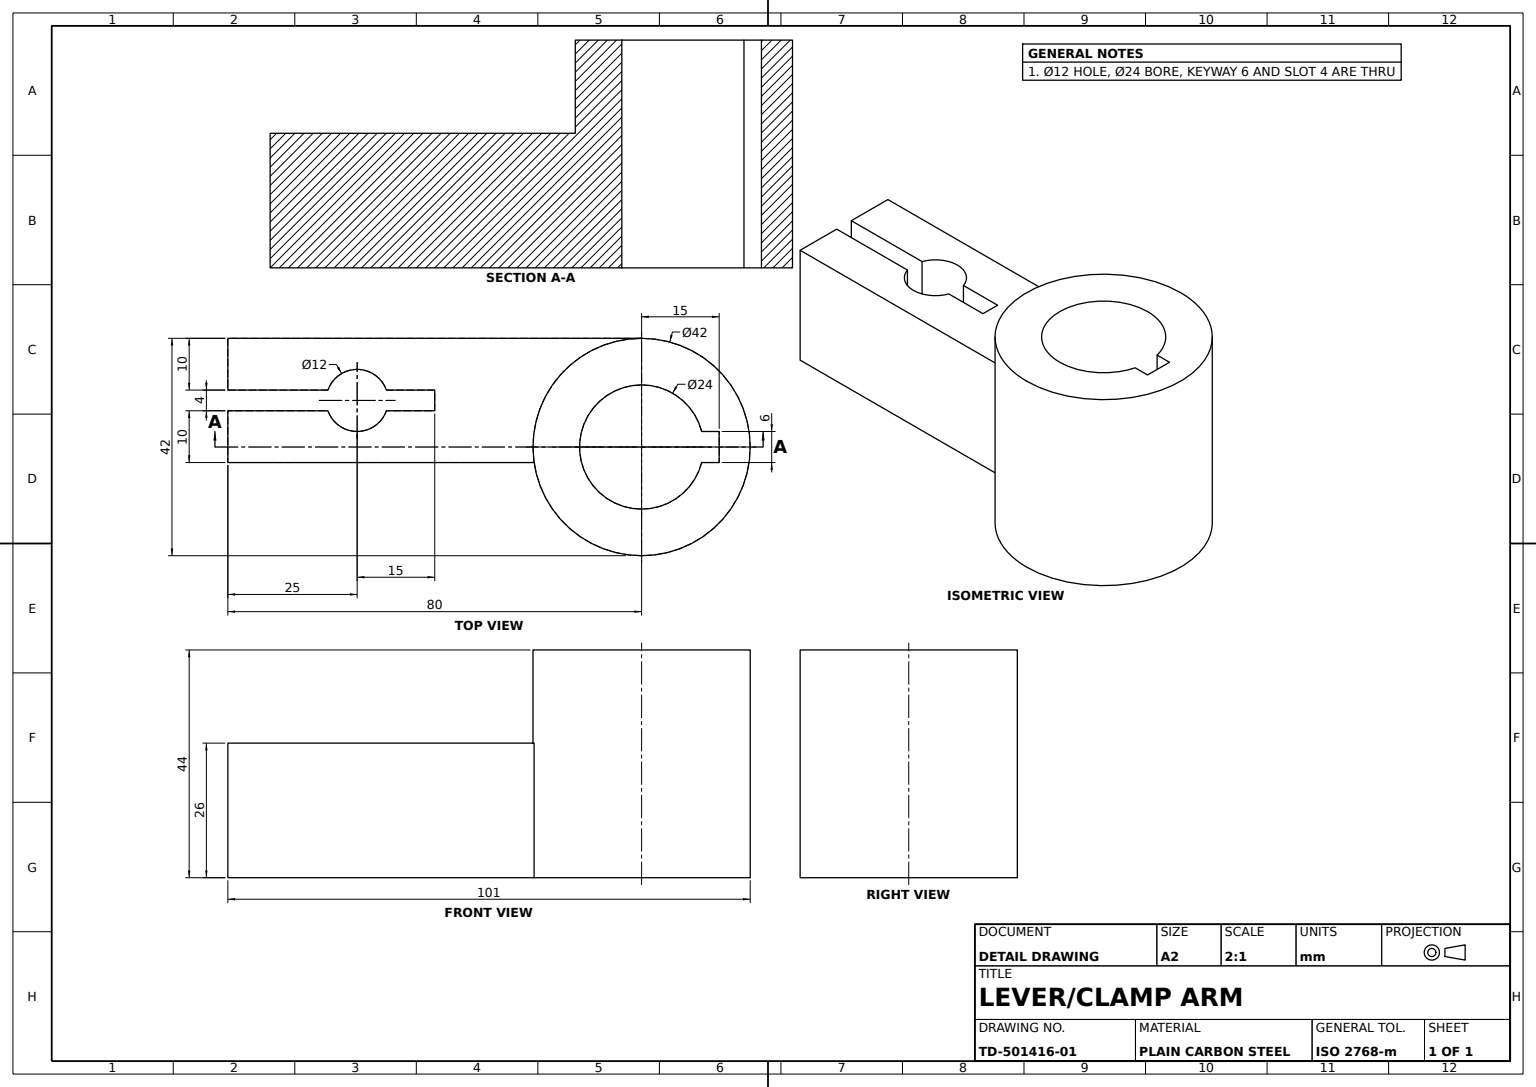
from build123d import *

# Parameters (mm, degrees)
LEVER_ARM_PROFILE_W        = 80
LEVER_ARM_PROFILE_H        = 26
LEVER_ARM_80X26_DEPTH      = 24
HUB_PROFILE_42_R           = 21
HUB_BOSS_42_DEPTH          = 26
HUB_START                  = 18
HUB_EXTENSION_PROFILE_42_R = 21
HUB_EXTENSION_42_DEPTH     = 18
CLAMP_SPLIT_SLOT_DEPTH     = 30
KEYED_BORE_24_DEPTH        = 50


with BuildPart() as part:
    # Lever Arm Profile → Lever Arm 80x26 (new body)
    with BuildSketch(Plane.XY):
        with Locations((40, 13)):
            Rectangle(LEVER_ARM_PROFILE_W, LEVER_ARM_PROFILE_H)
    extrude(amount=-LEVER_ARM_80X26_DEPTH)

    # Hub Profile Ø42 → Hub Boss Ø42 (add)
    with BuildSketch(Plane(origin=(0, 26, 0), x_dir=(1, 0, 0), z_dir=(0, 1, 0))):
        with Locations((80, 3)):
            Circle(HUB_PROFILE_42_R)
    extrude(amount=-HUB_BOSS_42_DEPTH)

    # Hub Extension Profile Ø42 → Hub Extension Ø42 (add)
    with BuildSketch(Plane(origin=(0, 26, 0), x_dir=(1, 0, 0), z_dir=(0, 1, 0)).offset(HUB_START)):
        with Locations(Location((80, 3, 0), (0, 0, 270))):
            Circle(HUB_EXTENSION_PROFILE_42_R)
    extrude(amount=-HUB_EXTENSION_42_DEPTH)

    # Clamp Slot Profile → Clamp Split Slot (cut)
    with BuildSketch(Plane(origin=(0, 26, 0), x_dir=(1, 0, 0), z_dir=(0, 1, 0))):
        with BuildLine():
            Line((0, 14), (0, 10))
            Line((0, 10), (19.343145751, 10))
            ThreePointArc((19.343145751, 10), (25, 6), (30.656854249, 10))
            Line((30.656854249, 10), (40, 10))
            Line((40, 10), (40, 14))
            Line((40, 14), (30.656854249, 14))
            ThreePointArc((30.656854249, 14), (25, 18), (19.343145751, 14))
            Line((19.343145751, 14), (0, 14))
        make_face()
    extrude(amount=-CLAMP_SPLIT_SLOT_DEPTH, mode=Mode.SUBTRACT)

    # Keyed Bore Profile → Keyed Bore Ø24 (cut)
    with BuildSketch(Plane(origin=(0, 44, 0), x_dir=(1, 0, 0), z_dir=(0, 1, 0))):
        with BuildLine():
            Line((95, 6), (91.618950039, 6))
            ThreePointArc((91.618950039, 6), (68, 3), (91.618950039, 0))
            Line((91.618950039, 0), (95, 0))
            Line((95, 0), (95, 6))
        make_face()
    extrude(amount=-KEYED_BORE_24_DEPTH, mode=Mode.SUBTRACT)


solid = part.part
